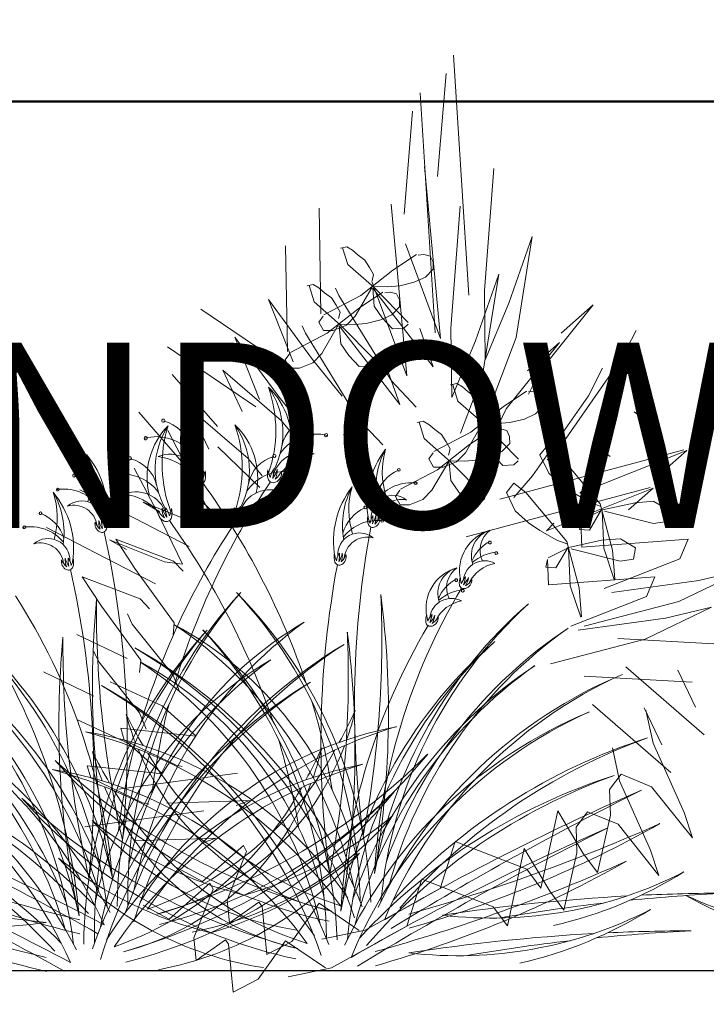
# Model space of a CAD drawing. Units: inches. Extents: x 89 to 490, y -59 to 378.
# Tile 10 of 20: x 352 to 374, y -24 to 7. Entities that reach past the tile are written whole.
import ezdxf

# ---------------------------------------------------------------- set-up
doc = ezdxf.new("R2010")
doc.units = ezdxf.units.IN
doc.header["$MEASUREMENT"] = 0
for name, color, linetype, lineweight in [('A-ANNO-DIMS', 2, 'Continuous', 18), ('L-PLNT', 94, 'Continuous', 18), ('L-PLNT-EDGE', 31, 'Continuous', 25), ('Outer Walls', 12, 'Continuous', 50), ('Windows', 171, 'Continuous', 25)]:
    doc.layers.add(name, color=color, linetype=linetype, lineweight=lineweight)
doc.layers.add('fl', color=73, linetype='Continuous', lineweight=9, true_color=0xa3d166)
doc.styles.get("Standard").update_dxf_attribs({"font": 'arial.ttf'})
doc.dimstyles.get("Standard").update_dxf_attribs({"dimtxt": 6, "dimasz": 4, "dimexe": 3, "dimexo": 3, "dimgap": 0.09, "dimtad": 0, "dimtih": 1, "dimtoh": 1, "dimdec": 1, "dimzin": 0, "dimdsep": 46, "dimlunit": 3, "dimtxsty": 'Standard', "dimcen": 0.09, "dimadec": 0, "dimazin": 0, "dimtfac": 1, "dimtdec": 1, "dimtofl": 0, "dimtmove": 0, "dimatfit": 3, "dimfxl": 1, "dimtolj": 1, "dimtzin": 0, "dimarcsym": 0})

# ---------------------------------------------------------------- blocks, each defined once
blk = doc.blocks.new('Window')
blk.add_lwpolyline([(588.369, 99.053), (588.369, 90.053), (516.369, 90.053), (516.369, 99.053)], close=True)
blk = doc.blocks.new('Plantation')
at = {"layer": 'fl'}
for p, q in [((590.053, 41.103), (590.545, 33.342)), ((589.537, 37.183), (589.811, 40.515)), ((588.969, 39.885), (589.462, 32.124)), ((588.453, 35.965), (588.728, 39.297)), ((589.116, 37.508), (589.628, 31.944)), ((591.356, 37.436), (591.053, 33.489)), ((585.761, 32.741), (585.701, 36.153)), ((588.032, 36.29), (588.545, 30.726)), ((590.272, 36.218), (589.969, 32.271)), ((591.845, 33.078), (592.598, 35.243)), ((592.598, 35.243), (592.077, 31.968)), ((584.677, 31.523), (584.617, 34.935)), ((586.397, 34.862), (586.597, 34.902)), ((586.465, 34.869), (586.629, 34.339)), ((586.597, 34.902), (586.781, 34.796)), ((586.781, 34.796), (586.965, 34.635)), ((589.628, 31.944), (588.494, 35.002)), ((586.965, 34.635), (587.187, 34.475)), ((587.187, 34.475), (587.336, 34.241)), ((588.094, 34.146), (588.854, 34.658)), ((589.094, 34.654), (588.912, 34.633)), ((589.295, 34.603), (589.094, 34.654)), ((589.389, 34.405), (589.295, 34.603)), ((586.629, 34.339), (587.481, 33.591)), ((587.052, 33.333), (588.094, 34.146)), ((587.336, 34.241), (587.468, 34.007)), ((589.143, 33.927), (589.393, 34.186)), ((589.393, 34.186), (589.389, 34.405)), ((588.545, 30.726), (587.411, 33.784)), ((587.468, 34.007), (587.417, 33.806)), ((588.782, 33.757), (589.143, 33.927)), ((590.761, 31.86), (591.514, 34.025)), ((591.514, 34.025), (590.994, 30.75)), ((585.314, 33.644), (585.513, 33.684)), ((585.381, 33.651), (585.545, 33.121)), ((585.513, 33.684), (585.697, 33.578)), ((585.697, 33.578), (585.882, 33.417)), ((586.238, 33.567), (586.343, 33.328)), ((586.872, 32.667), (587.42, 33.605)), ((587.439, 33.569), (589.395, 31.025)), ((587.439, 33.569), (587.485, 32.988)), ((587.474, 33.625), (587.929, 33.614)), ((587.481, 33.591), (588.589, 32.462)), ((587.929, 33.614), (588.311, 33.639)), ((588.311, 33.639), (588.782, 33.757)), ((591.053, 33.489), (591.081, 31.253)), ((584.861, 31.187), (584.063, 33.202)), ((584.063, 33.202), (585.49, 31.257)), ((585.858, 32.709), (587.052, 33.333)), ((585.882, 33.417), (586.103, 33.257)), ((586.103, 33.257), (586.252, 33.023)), ((586.343, 33.328), (588.042, 30.566)), ((587.01, 32.928), (587.77, 33.44)), ((588.01, 33.436), (587.828, 33.415)), ((588.211, 33.385), (588.01, 33.436)), ((588.305, 33.187), (588.211, 33.385)), ((588.309, 32.968), (588.305, 33.187)), ((584.741, 30.944), (581.881, 32.89)), ((585.545, 33.121), (586.397, 32.373)), ((585.968, 32.115), (587.01, 32.928)), ((586.252, 33.023), (586.384, 32.789)), ((587.485, 32.988), (587.747, 32.61)), ((588.059, 32.709), (588.309, 32.968)), ((591.081, 31.253), (591.845, 33.078)), ((594.569, 33.025), (592.844, 30.876)), ((593.531, 32.115), (594.569, 33.025)), ((585.835, 32.667), (585.693, 32.465)), ((586.384, 32.789), (586.333, 32.588)), ((586.587, 32.371), (586.872, 32.667)), ((587.227, 32.421), (587.698, 32.539)), ((587.698, 32.539), (588.059, 32.709)), ((587.747, 32.61), (588.08, 32.251)), ((585.154, 32.349), (585.259, 32.11)), ((585.693, 32.465), (585.844, 32.194)), ((585.789, 31.449), (586.336, 32.387)), ((585.844, 32.194), (586.153, 32.199)), ((586.153, 32.199), (586.587, 32.371)), ((586.355, 32.351), (588.311, 29.807)), ((586.355, 32.351), (586.402, 31.77)), ((586.39, 32.407), (586.845, 32.396)), ((586.397, 32.373), (587.505, 31.244)), ((586.845, 32.396), (587.227, 32.421)), ((588.08, 32.251), (588.444, 32.276)), ((588.444, 32.276), (588.587, 32.406)), ((589.395, 31.025), (588.958, 32.265)), ((589.969, 32.271), (589.997, 30.035)), ((595.959, 32.197), (595.503, 31.307)), ((583.777, 29.969), (582.979, 31.984)), ((582.979, 31.984), (584.406, 30.039)), ((584.774, 31.491), (585.968, 32.115)), ((585.259, 32.11), (586.958, 29.348)), ((592.077, 31.968), (591.363, 30.096)), ((583.658, 29.726), (580.797, 31.672)), ((586.402, 31.77), (586.663, 31.392)), ((589.997, 30.035), (590.761, 31.86)), ((593.485, 31.807), (591.76, 29.658)), ((592.447, 30.897), (593.485, 31.807)), ((584.752, 31.449), (584.61, 31.247)), ((584.61, 31.247), (584.76, 30.976)), ((585.49, 31.257), (586.454, 30.075)), ((585.503, 31.153), (585.789, 31.449)), ((586.663, 31.392), (586.997, 31.033)), ((595.503, 31.307), (593.695, 28.717)), ((583.214, 29.575), (582.585, 30.915)), ((582.585, 30.915), (584.488, 29.278)), ((584.76, 30.976), (585.069, 30.981)), ((585.069, 30.981), (585.503, 31.153)), ((586.997, 31.033), (587.36, 31.058)), ((587.36, 31.058), (587.503, 31.188)), ((588.311, 29.807), (587.874, 31.047)), ((594.875, 30.979), (594.419, 30.089)), ((580.949, 30.771), (582.414, 29.091)), ((590.994, 30.75), (590.28, 28.878)), ((592.844, 30.876), (592.48, 30.134)), ((588.042, 30.566), (588.848, 29.719)), ((589.96, 30.439), (590.159, 30.479)), ((590.027, 30.445), (590.191, 29.916)), ((590.159, 30.479), (590.343, 30.373)), ((590.343, 30.373), (590.528, 30.212)), ((584.406, 30.039), (585.37, 28.857)), ((590.528, 30.212), (590.749, 30.052)), ((590.749, 30.052), (590.898, 29.818)), ((591.656, 29.723), (592.416, 30.235)), ((592.656, 30.231), (592.474, 30.21)), ((594.419, 30.089), (592.611, 27.499)), ((592.857, 30.18), (592.656, 30.231)), ((592.951, 29.982), (592.857, 30.18)), ((592.955, 29.763), (592.951, 29.982)), ((582.13, 28.357), (581.501, 29.697)), ((581.501, 29.697), (583.404, 28.06)), ((590.191, 29.916), (591.043, 29.168)), ((590.614, 28.91), (591.656, 29.723)), ((590.898, 29.818), (591.03, 29.584)), ((591.76, 29.658), (591.396, 28.916)), ((592.705, 29.504), (592.955, 29.763)), ((579.865, 29.553), (581.33, 27.873)), ((586.958, 29.348), (587.765, 28.501)), ((591.03, 29.584), (590.979, 29.383)), ((591.873, 29.216), (592.344, 29.334)), ((592.344, 29.334), (592.705, 29.504)), ((595.902, 29.57), (596.202, 29.338)), ((584.488, 29.278), (584.945, 28.711)), ((588.876, 29.221), (589.075, 29.261)), ((588.943, 29.227), (589.107, 28.698)), ((589.075, 29.261), (589.259, 29.155)), ((589.259, 29.155), (589.444, 28.994)), ((589.444, 28.994), (589.665, 28.834)), ((590.435, 28.244), (590.982, 29.182)), ((590.572, 28.505), (591.332, 29.017)), ((591.001, 29.146), (591.048, 28.564)), ((591.036, 29.202), (591.491, 29.191)), ((591.043, 29.168), (592.151, 28.039)), ((591.572, 29.013), (591.39, 28.992)), ((591.491, 29.191), (591.873, 29.216)), ((591.773, 28.962), (591.572, 29.013)), ((581.532, 27.573), (580.805, 28.958)), ((589.107, 28.698), (589.959, 27.95)), ((589.42, 28.286), (590.614, 28.91)), ((589.665, 28.834), (589.814, 28.6)), ((591.867, 28.764), (591.773, 28.962)), ((591.871, 28.545), (591.867, 28.764)), ((593.695, 28.717), (593.087, 28.016)), ((582.427, 28.43), (583.784, 27.115)), ((589.53, 27.692), (590.572, 28.505)), ((589.814, 28.6), (589.946, 28.366)), ((589.946, 28.366), (589.895, 28.165)), ((591.048, 28.564), (591.309, 28.187)), ((591.621, 28.286), (591.871, 28.545)), ((592.85, 28.177), (593.091, 28.479)), ((593.091, 28.479), (593.481, 28.173)), ((583.404, 28.06), (583.861, 27.493)), ((589.398, 28.244), (589.256, 28.042)), ((589.256, 28.042), (589.406, 27.771)), ((590.149, 27.948), (590.435, 28.244)), ((590.789, 27.998), (591.26, 28.116)), ((591.26, 28.116), (591.621, 28.286)), ((591.309, 28.187), (591.643, 27.828)), ((597.505, 28.338), (591.548, 26.737)), ((593.134, 27.583), (592.85, 28.177)), ((594.798, 26.589), (593.475, 28.174)), ((594.145, 26.934), (597.598, 28.316)), ((594.818, 28.352), (595.118, 28.12)), ((597.598, 28.316), (596.796, 27.608)), ((580.449, 26.355), (579.721, 27.74)), ((589.351, 27.026), (589.898, 27.964)), ((589.406, 27.771), (589.715, 27.776)), ((589.715, 27.776), (590.149, 27.948)), ((589.917, 27.928), (589.964, 27.346)), ((589.953, 27.984), (590.408, 27.973)), ((589.959, 27.95), (591.067, 26.821)), ((590.408, 27.973), (590.789, 27.998)), ((591.643, 27.828), (592.006, 27.853)), ((592.006, 27.853), (592.149, 27.983)), ((582.369, 25.852), (581.532, 27.573)), ((588.336, 27.068), (589.53, 27.692)), ((592.611, 27.499), (592.003, 26.798)), ((593.56, 27.19), (593.134, 27.583)), ((581.343, 27.212), (582.7, 25.897)), ((589.964, 27.346), (590.225, 26.969)), ((596.421, 27.12), (590.464, 25.519)), ((591.766, 26.959), (592.007, 27.261)), ((592.007, 27.261), (592.397, 26.955)), ((593.061, 25.716), (596.514, 27.098)), ((593.934, 26.948), (593.56, 27.19)), ((594.379, 27.185), (594.145, 26.934)), ((596.514, 27.098), (595.712, 26.39)), ((581.495, 25.213), (577.963, 27.037)), ((588.314, 27.026), (588.172, 26.824)), ((588.172, 26.824), (588.322, 26.553)), ((589.065, 26.73), (589.351, 27.026)), ((590.225, 26.969), (590.559, 26.61)), ((590.922, 26.635), (591.065, 26.765)), ((592.05, 26.365), (591.766, 26.959)), ((593.714, 25.371), (592.391, 26.956)), ((594.479, 26.634), (593.934, 26.948)), ((580.554, 26.325), (580.008, 26.646)), ((580.008, 26.646), (581.783, 25.929)), ((588.322, 26.553), (588.631, 26.558)), ((588.631, 26.558), (589.065, 26.73)), ((590.559, 26.61), (590.922, 26.635)), ((594.803, 26.513), (594.479, 26.634)), ((595.202, 25.087), (594.798, 26.589)), ((595.927, 26.626), (594.873, 26.397)), ((596.534, 26.679), (595.927, 26.626)), ((596.536, 26.669), (597.02, 26.38)), ((581.285, 24.634), (580.449, 26.355)), ((592.476, 25.972), (592.05, 26.365)), ((594.873, 26.397), (594.195, 26.057)), ((594.451, 25.739), (594.846, 26.409)), ((594.913, 25.157), (594.86, 26.374)), ((596.526, 25.953), (594.938, 26.356)), ((597.02, 26.38), (596.956, 26.019)), ((580.411, 23.995), (576.879, 25.819)), ((581.783, 25.929), (582.369, 25.852)), ((592.85, 25.73), (592.476, 25.972)), ((593.296, 25.967), (593.061, 25.716)), ((594.176, 26.011), (594.128, 25.758)), ((594.176, 26.011), (594.205, 25.186)), ((596.956, 26.019), (596.526, 25.953)), ((593.395, 25.416), (592.85, 25.73)), ((594.128, 25.758), (594.451, 25.739)), ((579.47, 25.107), (578.925, 25.428)), ((578.925, 25.428), (580.699, 24.711)), ((579.741, 24.498), (579.126, 25.45)), ((579.126, 25.45), (580.997, 24.736)), ((593.789, 25.179), (593.111, 24.839)), ((593.367, 24.521), (593.762, 25.191)), ((593.719, 25.295), (593.395, 25.416)), ((594.119, 23.869), (593.714, 25.371)), ((594.844, 25.408), (593.789, 25.179)), ((594.205, 25.186), (597.647, 25.449)), ((595.45, 25.461), (594.844, 25.408)), ((595.452, 25.451), (595.936, 25.162)), ((597.647, 25.449), (597.377, 24.808)), ((593.83, 23.939), (593.776, 25.156)), ((595.442, 24.735), (593.855, 25.138)), ((595.251, 24.138), (594.913, 25.157)), ((595.273, 24.155), (595.202, 25.087)), ((595.936, 25.162), (595.872, 24.801)), ((580.699, 24.711), (581.285, 24.634)), ((580.997, 24.736), (581.3, 24.406)), ((593.093, 24.793), (593.044, 24.54)), ((593.044, 24.54), (593.367, 24.521)), ((593.093, 24.793), (593.121, 23.968)), ((597.377, 24.808), (594.931, 23.85)), ((595.872, 24.801), (595.442, 24.735)), ((578.658, 23.28), (578.042, 24.232)), ((578.042, 24.232), (579.913, 23.518)), ((581.017, 22.743), (579.741, 24.498)), ((593.121, 23.968), (596.563, 24.231)), ((596.563, 24.231), (596.293, 23.59)), ((599.485, 24.463), (597.342, 23.428)), ((597.995, 24.105), (599.485, 24.463)), ((594.167, 22.92), (593.83, 23.939)), ((595.175, 23.723), (597.995, 24.105)), ((596.293, 23.59), (593.847, 22.632)), ((594.189, 22.937), (594.119, 23.869)), ((579.933, 21.525), (578.658, 23.28)), ((579.913, 23.518), (580.216, 23.188)), ((597.342, 23.428), (594.28, 22.626)), ((579.657, 22.697), (579.5, 23.032)), ((598.401, 23.245), (596.258, 22.21)), ((596.911, 22.887), (598.401, 23.245)), ((580.977, 21.04), (579.657, 22.697)), ((580.981, 22.353), (581.017, 22.743)), ((594.091, 22.505), (596.911, 22.887)), ((577.865, 22.366), (579.494, 21.586)), ((596.258, 22.21), (593.196, 21.408)), ((595.368, 22.229), (598.862, 22.04)), ((578.573, 21.479), (578.416, 21.814)), ((579.894, 19.822), (578.573, 21.479)), ((579.897, 21.135), (579.933, 21.525)), ((576.781, 21.148), (578.41, 20.368)), ((581.19, 20.513), (580.977, 21.04)), ((595.633, 21.318), (598.165, 19.117)), ((597.306, 21.208), (597.881, 20.013)), ((580.622, 20.056), (578.943, 20.825)), ((594.284, 21.011), (597.778, 20.822)), ((594.549, 20.1), (597.081, 17.899)), ((580.106, 19.295), (579.894, 19.822)), ((581.725, 19.073), (580.622, 20.056)), ((596.222, 19.99), (596.797, 18.795)), ((596.28, 19.909), (596.511, 18.848)), ((579.538, 18.838), (577.859, 19.607)), ((579.396, 18.945), (579.286, 19.33)), ((579.286, 19.33), (580.993, 19.145)), ((580.993, 19.145), (581.725, 19.073)), ((581.077, 18.127), (579.396, 18.945)), ((580.641, 17.855), (579.538, 18.838)), ((596.511, 18.848), (597.511, 16.597)), ((595.196, 18.691), (595.427, 17.63)), ((578.312, 17.727), (578.202, 18.112)), ((578.202, 18.112), (579.91, 17.927)), ((579.208, 17.36), (583.059, 17.877)), ((579.91, 17.927), (580.641, 17.855)), ((581.273, 18.085), (581.077, 18.127)), ((579.993, 16.909), (578.312, 17.727)), ((595.476, 17.84), (595.104, 17.341)), ((595.427, 17.63), (596.428, 15.379)), ((596.462, 17.436), (595.476, 17.84)), ((595.104, 17.341), (595.132, 16.516)), ((597.782, 15.78), (596.462, 17.436)), ((580.189, 16.867), (579.993, 16.909)), ((582.478, 16.96), (580.778, 16.902)), ((583.449, 16.993), (582.478, 16.96)), ((583.017, 16.832), (583.449, 16.993)), ((578.125, 16.142), (581.975, 16.659)), ((593.426, 16.652), (592.879, 14.154)), ((594.251, 15.271), (593.426, 16.652)), ((594.392, 16.622), (594.02, 16.123)), ((595.378, 16.218), (594.392, 16.622)), ((597.511, 16.597), (597.782, 15.78)), ((595.132, 16.516), (594.709, 14.654)), ((594.02, 16.123), (594.048, 15.298)), ((596.698, 14.562), (595.378, 16.218)), ((581.394, 15.741), (579.694, 15.684)), ((582.365, 15.775), (581.394, 15.741)), ((581.933, 15.614), (582.365, 15.775)), ((590.105, 15.664), (589.623, 14.141)), ((592.421, 14.771), (590.105, 15.664)), ((583.256, 15.528), (581.934, 14.365)), ((582.733, 13.76), (583.359, 15.337)), ((583.359, 15.337), (583.256, 15.528)), ((592.342, 15.434), (591.795, 12.936)), ((593.167, 14.053), (592.342, 15.434)), ((594.048, 15.298), (593.626, 13.436)), ((596.428, 15.379), (596.698, 14.562)), ((594.709, 14.654), (594.251, 15.271)), ((581.934, 14.365), (581.092, 14.822)), ((592.879, 14.154), (592.421, 14.771)), ((589.022, 14.446), (588.539, 12.923)), ((591.337, 13.553), (589.022, 14.446)), ((582.172, 14.31), (580.85, 13.146)), ((581.649, 12.542), (582.276, 14.119)), ((582.276, 14.119), (582.172, 14.31)), ((589.623, 14.141), (587.189, 12.794)), ((593.626, 13.436), (593.167, 14.053)), ((582.806, 13.033), (582.733, 13.76)), ((580.85, 13.146), (580.008, 13.604)), ((583.756, 13.697), (582.806, 13.033)), ((583.858, 13.555), (583.756, 13.697)), ((584.008, 12.005), (583.858, 13.555)), ((585.701, 13.667), (584.82, 12.421)), ((586.995, 12.787), (585.701, 13.667)), ((591.795, 12.936), (591.337, 13.553)), ((587.189, 12.794), (585.79, 12.503)), ((588.539, 12.923), (586.106, 11.576)), ((581.722, 11.815), (581.649, 12.542)), ((582.672, 12.479), (581.722, 11.815)), ((582.774, 12.337), (582.672, 12.479)), ((584.617, 12.449), (583.736, 11.203)), ((585.911, 11.569), (584.617, 12.449)), ((582.924, 10.787), (582.774, 12.337)), ((584.82, 12.421), (584.008, 12.005)), ((586.106, 11.576), (584.706, 11.285)), ((583.736, 11.203), (582.924, 10.787))]:
    blk.add_line(p, q, dxfattribs=at)
for centre, radius, start, end in [((583.596, 28.668), 2.375, 135.5632, 193.7293), ((584.084, 28.918), 2.601, 147.096, 209.2874), ((585.935, 29.073), 4.227, 162.6858, 201.1197), ((581.93, 28.875), 2.601, 332.7126, 34.904), ((582.427, 28.642), 2.375, 348.2707, 46.4368), ((580.075, 28.965), 4.227, 340.8803, 19.3142), ((580.662, 29.279), 0.053, 11.802, 191.802), ((585.639, 28.222), 1.163, 105.8563, 168.2872), ((585.338, 29.356), 0.053, 350.198, 170.198), ((585.338, 29.356), 0.053, 170.198, 350.198), ((582.512, 27.45), 2.375, 135.5632, 193.7293), ((583, 27.7), 2.601, 147.096, 209.2874), ((580.662, 29.279), 0.053, 191.802, 11.802), ((584.851, 27.855), 4.227, 162.6858, 201.1197), ((580.4, 28.136), 1.163, 13.7128, 76.1437), ((580.847, 27.657), 2.601, 332.7126, 34.904), ((581.343, 27.424), 2.375, 348.2707, 46.4368), ((578.991, 27.747), 4.227, 340.8803, 19.3142), ((580.093, 28.713), 0.053, 11.802, 191.802), ((580.441, 27.347), 1.416, 35.6636, 106.404), ((580.093, 28.713), 0.053, 191.802, 11.802), ((585.626, 27.432), 1.416, 75.596, 146.3364), ((585.925, 28.809), 0.053, 170.198, 350.198), ((585.925, 28.809), 0.053, 350.198, 170.198), ((575.991, 26.352), 2.854, 351.4134, 39.8275), ((575.706, 27.362), 2.608, 344.3064, 18.279), ((575.935, 26.873), 2.6, 351.5096, 30.1949), ((579.578, 28.061), 0.053, 11.802, 191.802), ((579.578, 28.061), 0.053, 191.802, 11.802), ((579.316, 26.918), 1.163, 13.7128, 76.1437), ((580.873, 27.183), 1.01, 11.1862, 111.7493), ((580.216, 26.257), 1.886, 44.0209, 81.3627), ((584.555, 27.004), 1.163, 105.8563, 168.2872), ((584.254, 28.138), 0.053, 350.198, 170.198), ((584.254, 28.138), 0.053, 170.198, 350.198), ((585.199, 27.253), 1.01, 70.2507, 170.8138), ((585.889, 26.351), 1.886, 100.6373, 137.9791), ((590.108, 26.604), 2.854, 142.1725, 190.5866), ((590.145, 27.126), 2.6, 151.8051, 190.4904), ((590.357, 27.623), 2.608, 163.721, 197.6936), ((588.284, 27.691), 0.0459, 354.4108, 174.4108), ((577.775, 27.502), 0.0459, 7.5892, 187.5892), ((577.775, 27.502), 0.0459, 187.5892, 7.5892), ((577.34, 26.331), 1.243, 16.8512, 68.8014), ((579.009, 27.495), 0.053, 11.802, 191.802), ((579.357, 26.129), 1.416, 35.6636, 106.404), ((579.009, 27.495), 0.053, 191.802, 11.802), ((581.906, 27.557), 0.334, 172.3781, 246.6066), ((582.195, 27.901), 0.689, 205.7422, 233.1344), ((582.36, 27.654), 0.654, 178.723, 207.7572), ((582.516, 27.921), 0.848, 197.3111, 219.7508), ((581.179, 27.188), 0.803, 16.3461, 37.9549), ((583.321, 27.787), 1.513, 184.0141, 195.6693), ((580.816, 27.847), 1.213, 339.0728, 350.8866), ((581.342, 27.507), 0.688, 348.1534, 12.4334), ((584.542, 26.214), 1.416, 75.596, 146.3364), ((584.72, 27.56), 0.688, 169.5666, 193.8466), ((585.233, 27.919), 1.213, 191.1134, 202.9272), ((584.894, 27.247), 0.803, 144.0451, 165.6539), ((582.732, 27.772), 1.513, 346.3307, 357.9859), ((583.531, 27.933), 0.848, 322.2492, 344.6889), ((583.697, 27.672), 0.654, 334.2428, 3.277), ((583.853, 27.925), 0.689, 308.8656, 336.2578), ((584.154, 27.591), 0.334, 295.3934, 9.6219), ((584.841, 27.591), 0.053, 170.198, 350.198), ((584.841, 27.591), 0.053, 350.198, 170.198), ((588.76, 26.535), 1.243, 113.1986, 165.1488), ((588.284, 27.691), 0.0459, 174.4108, 354.4108), ((577.249, 27.05), 0.0459, 7.5892, 187.5892), ((604.656, 13.567), 24.696, 146.2244, 163.2125), ((581.846, 27.41), 0.175, 245.3588, 345.3239), ((561.906, 12.826), 24.696, 18.7875, 35.7756), ((584.219, 27.446), 0.175, 196.6761, 296.6412), ((589.024, 25.386), 2.854, 142.1725, 190.5866), ((589.061, 25.908), 2.6, 151.8051, 190.4904), ((589.273, 26.405), 2.608, 163.721, 197.6936), ((588.675, 25.883), 1.386, 81.8677, 142.4931), ((588.826, 27.257), 0.0459, 354.4108, 174.4108), ((588.826, 27.257), 0.0459, 174.4108, 354.4108), ((574.907, 25.134), 2.854, 351.4134, 39.8275), ((574.622, 26.144), 2.608, 344.3064, 18.279), ((574.851, 25.654), 2.6, 351.5096, 30.1949), ((577.447, 25.682), 1.386, 39.5069, 100.1323), ((577.249, 27.05), 0.0459, 187.5892, 7.5892), ((579.789, 25.965), 1.01, 11.1862, 111.7493), ((579.132, 25.039), 1.886, 44.0209, 81.3627), ((584.115, 26.035), 1.01, 70.2507, 170.8138), ((584.805, 25.132), 1.886, 100.6373, 137.9791), ((588.092, 26.164), 0.701, 51.1297, 184.5825), ((578.02, 25.984), 0.701, 357.4175, 130.8703), ((577.77, 25.789), 0.754, 6.9832, 106.1055), ((581.276, 26.436), 0.654, 178.723, 207.7572), ((581.432, 26.703), 0.848, 197.3111, 219.7508), ((580.095, 25.97), 0.803, 16.3461, 37.9549), ((582.237, 26.569), 1.513, 184.0141, 195.6693), ((583.636, 26.342), 0.688, 169.5666, 193.8466), ((584.149, 26.701), 1.213, 191.1134, 202.9272), ((583.81, 26.029), 0.803, 144.0451, 165.6539), ((581.648, 26.554), 1.513, 346.3307, 357.9859), ((582.448, 26.715), 0.848, 322.2492, 344.6889), ((582.613, 26.454), 0.654, 334.2428, 3.277), ((587.676, 25.317), 1.243, 113.1986, 165.1488), ((587.2, 26.473), 0.0459, 174.4108, 354.4108), ((587.2, 26.473), 0.0459, 354.4108, 174.4108), ((588.349, 25.979), 0.754, 75.8945, 175.0168), ((576.691, 26.284), 0.0459, 7.5892, 187.5892), ((576.691, 26.284), 0.0459, 187.5892, 7.5892), ((576.256, 25.113), 1.243, 16.8512, 68.8014), ((580.822, 26.339), 0.334, 172.3781, 246.6066), ((581.112, 26.683), 0.689, 205.7422, 233.1344), ((580.762, 26.192), 0.175, 245.3588, 345.3239), ((579.732, 26.629), 1.213, 339.0728, 350.8866), ((580.258, 26.289), 0.688, 348.1534, 12.4334), ((583.135, 26.228), 0.175, 196.6761, 296.6412), ((582.769, 26.707), 0.689, 308.8656, 336.2578), ((583.07, 26.373), 0.334, 295.3934, 9.6219), ((587.865, 26.103), 0.595, 173.7794, 198.0594), ((588.285, 26.445), 1.049, 195.3262, 207.14), ((588.035, 25.844), 0.694, 148.2579, 169.8667), ((586.138, 26.159), 1.308, 350.5435, 2.1987), ((586.817, 26.35), 0.733, 326.462, 348.9017), ((586.976, 26.135), 0.565, 338.4556, 7.4897), ((587.095, 26.363), 0.596, 313.0784, 340.4706), ((587.376, 26.094), 0.289, 299.6062, 13.8346), ((576.165, 25.832), 0.0459, 7.5892, 187.5892), ((576.363, 24.464), 1.386, 39.5069, 100.1323), ((576.165, 25.832), 0.0459, 187.5892, 7.5892), ((578.739, 25.938), 0.289, 168.1654, 242.3938), ((579.01, 26.216), 0.596, 201.5294, 228.9216), ((579.137, 25.993), 0.565, 174.5103, 203.5444), ((579.288, 26.213), 0.733, 193.0983, 215.538), ((579.974, 26.047), 1.308, 179.8013, 191.4565), ((578.088, 25.666), 0.694, 12.1333, 33.7421), ((577.817, 26.257), 1.049, 334.86, 346.6738), ((578.249, 25.93), 0.595, 343.9406, 8.2206), ((603.572, 12.349), 24.696, 146.2244, 163.2125), ((560.822, 11.608), 24.696, 18.7875, 35.7756), ((587.591, 24.665), 1.386, 81.8677, 142.4931), ((618.338, 20.073), 31.492, 169.4573, 187.7209), ((587.441, 25.973), 0.151, 200.8889, 300.854), ((587.742, 26.039), 0.0459, 354.4108, 174.4108), ((587.742, 26.039), 0.0459, 174.4108, 354.4108), ((578.678, 25.815), 0.151, 241.146, 341.1111), ((548.006, 18.841), 31.492, 354.2791, 12.5427), ((587.008, 24.946), 0.701, 51.1297, 184.5825), ((587.265, 24.761), 0.754, 75.8945, 175.0168), ((591.615, 24.421), 1.368, 105.8634, 192.367), ((591.493, 24.911), 0.863, 106.9799, 199.184), ((591.704, 25.093), 0.793, 125.7722, 206.2024), ((576.936, 24.766), 0.701, 357.4175, 130.8703), ((576.687, 24.571), 0.754, 6.9832, 106.1055), ((591.8, 24.269), 1.243, 116.6992, 157.9158), ((591.227, 25.335), 0.0459, 162.351, 342.351), ((591.227, 25.335), 0.0459, 342.351, 162.351), ((586.781, 24.885), 0.595, 173.7794, 198.0594), ((587.202, 25.227), 1.049, 195.3262, 207.14), ((586.951, 24.626), 0.694, 148.2579, 169.8667), ((585.054, 24.941), 1.308, 350.5435, 2.1987), ((585.733, 25.132), 0.733, 326.462, 348.9017), ((585.892, 24.917), 0.565, 338.4556, 7.4897), ((586.011, 25.145), 0.596, 313.0784, 340.4706), ((586.292, 24.876), 0.289, 299.6062, 13.8346), ((591.58, 23.649), 1.386, 94.6451, 131.584), ((591.438, 24.996), 0.0459, 162.351, 342.351), ((591.438, 24.996), 0.0459, 342.351, 162.351), ((577.655, 24.72), 0.289, 168.1654, 242.3938), ((577.927, 24.998), 0.596, 201.5294, 228.9216), ((578.053, 24.775), 0.565, 174.5103, 203.5444), ((578.204, 24.995), 0.733, 193.0983, 215.538), ((577.594, 24.597), 0.151, 241.146, 341.1111), ((578.89, 24.829), 1.308, 179.8013, 191.4565), ((577.005, 24.448), 0.694, 12.1333, 33.7421), ((576.734, 25.039), 1.049, 334.86, 346.6738), ((577.165, 24.712), 0.595, 343.9406, 8.2206), ((617.254, 18.855), 31.492, 169.4573, 187.7209), ((586.357, 24.755), 0.151, 200.8889, 300.854), ((591.064, 24.05), 0.696, 61.775, 172.7958), ((591.598, 23.527), 1.154, 100.1929, 154.0707), ((546.922, 17.622), 31.492, 354.2791, 12.5427), ((590.531, 23.203), 1.368, 105.8634, 192.367), ((590.409, 23.693), 0.863, 106.9799, 199.184), ((590.621, 23.875), 0.793, 125.7722, 206.2024), ((590.834, 24.033), 0.595, 161.7196, 185.9995), ((591.316, 24.28), 1.049, 183.2663, 195.0802), ((590.946, 23.745), 0.694, 136.198, 157.8068), ((589.157, 24.449), 1.308, 338.4836, 350.1389), ((590.716, 23.051), 1.243, 116.6992, 157.9158), ((590.143, 24.117), 0.0459, 162.351, 342.351), ((590.143, 24.117), 0.0459, 342.351, 162.351), ((590.392, 23.994), 0.151, 188.8291, 288.7942), ((589.86, 24.493), 0.733, 314.4022, 336.8418), ((590.354, 24.127), 0.289, 287.5463, 1.7748), ((589.971, 24.25), 0.565, 326.3958, 355.4299), ((590.135, 24.448), 0.596, 301.0185, 328.4108), ((558.885, 12.66), 20.216, 5.151, 32.7872), ((594.374, 13.451), 15.201, 137.4916, 179.6099), ((594.436, 13.941), 14.921, 139.0392, 181.297), ((572.107, 13.556), 14.921, 0.703, 42.9608), ((572.186, 13.068), 15.201, 2.3901, 44.5084), ((553.743, 22.201), 33.989, 349.2183, 2.4529), ((607.681, 13.517), 20.216, 149.2128, 176.849), ((558.054, 19.814), 29.894, 350.0105, 7.3826), ((590.497, 22.431), 1.386, 94.6451, 131.584), ((590.354, 23.777), 0.0459, 162.351, 342.351), ((590.354, 23.777), 0.0459, 342.351, 162.351), ((608.262, 20.685), 29.894, 174.6174, 191.9895), ((612.487, 23.221), 33.989, 179.5471, 192.7817), ((602.446, 11.881), 15.201, 130.9977, 169.5878), ((602.563, 12.361), 14.921, 132.5453, 174.8032), ((589.981, 22.832), 0.696, 61.775, 172.7958), ((590.514, 22.309), 1.154, 100.1929, 154.0707), ((564.04, 11.683), 14.921, 7.1968, 49.4547), ((564.174, 11.208), 15.201, 12.4122, 51.0023), ((589.75, 22.815), 0.595, 161.7196, 185.9995), ((590.233, 23.062), 1.049, 183.2663, 195.0802), ((589.862, 22.527), 0.694, 136.198, 157.8068), ((588.073, 23.231), 1.308, 338.4836, 350.1389), ((588.777, 23.275), 0.733, 314.4022, 336.8418), ((588.887, 23.032), 0.565, 326.3958, 355.4299), ((591.294, 12.388), 12.017, 120.3536, 167.8423), ((593.323, 11.517), 13.856, 125.7805, 169.1581), ((573.304, 11.172), 13.856, 12.8419, 56.2195), ((575.301, 12.114), 12.017, 14.1577, 61.6464), ((606.597, 12.299), 20.216, 149.2128, 176.849), ((589.308, 22.776), 0.151, 188.8291, 288.7942), ((589.27, 22.909), 0.289, 287.5463, 1.7748), ((589.051, 23.23), 0.596, 301.0185, 328.4108), ((557.801, 11.442), 20.216, 5.151, 32.7872), ((593.29, 12.232), 15.201, 137.4916, 179.6099), ((593.352, 12.723), 14.921, 139.0392, 181.297), ((571.023, 12.338), 14.921, 0.703, 42.9608), ((571.102, 11.85), 15.201, 2.3901, 44.5084), ((552.659, 20.983), 33.989, 349.2183, 2.4529), ((556.97, 18.596), 29.894, 350.0105, 7.3826), ((602.203, 9.926), 15.201, 123.7186, 160.4349), ((602.38, 10.388), 14.921, 125.2661, 165.1679), ((564.292, 9.718), 14.921, 16.8321, 56.7339), ((564.484, 9.263), 15.201, 21.5651, 58.2814), ((607.178, 19.467), 29.894, 174.6174, 191.9895), ((611.403, 22.003), 33.989, 179.5471, 192.7817), ((595.117, 7.795), 16.642, 121.1471, 160.292), ((595.251, 8.353), 16.239, 122.567, 163.1344), ((601.362, 10.663), 15.201, 130.9977, 169.5878), ((601.479, 11.143), 14.921, 132.5453, 174.8032), ((562.957, 10.465), 14.921, 7.1968, 49.4547), ((563.09, 9.99), 15.201, 12.4122, 51.0023), ((571.64, 7.391), 16.642, 21.708, 60.8529), ((571.487, 7.943), 16.239, 18.8656, 59.433), ((590.21, 11.17), 12.017, 120.3536, 167.8423), ((592.239, 10.299), 13.856, 125.7805, 169.1581), ((572.22, 9.954), 13.856, 12.8419, 56.2195), ((574.217, 10.896), 12.017, 14.1577, 61.6464), ((601.12, 8.708), 15.201, 123.7186, 160.4349), ((601.296, 9.17), 14.921, 125.2661, 165.1679), ((601.359, 7.034), 15.201, 112.5744, 154.7193), ((601.621, 7.453), 14.921, 114.122, 157.6363), ((563.208, 8.5), 14.921, 16.8321, 56.7339), ((563.401, 8.045), 15.201, 21.5651, 58.2814), ((594.034, 6.577), 16.642, 121.1471, 160.292), ((594.167, 7.135), 16.239, 122.567, 163.1344), ((565.43, 6.402), 15.201, 27.2807, 69.4256), ((565.153, 6.811), 14.921, 24.3637, 67.878), ((570.556, 6.173), 16.642, 21.708, 60.8529), ((570.404, 6.725), 16.239, 18.8656, 59.433), ((602.195, 14.513), 22.067, 165.3183, 172.932), ((564.333, 13.858), 22.067, 9.068, 16.6817), ((588.037, 22.079), 8.88, 194.9574, 201.3849), ((591.138, 25.442), 12.977, 205.8333, 210.9541), ((575.002, 25.155), 12.977, 331.0459, 336.1667), ((600.275, 5.816), 15.201, 112.5744, 154.7193), ((578.218, 21.902), 8.88, 340.6151, 347.0426), ((600.537, 6.235), 14.921, 114.122, 157.6363), ((564.346, 5.184), 15.201, 27.2807, 69.4256), ((564.069, 5.593), 14.921, 24.3637, 67.878), ((576.177, 6.722), 12.64, 34.1912, 81.04), ((574.36, 4.785), 14.911, 36.1662, 75.2917), ((590.606, 6.968), 12.64, 100.96, 147.8088), ((592.49, 5.097), 14.911, 106.7083, 145.8338), ((601.111, 13.295), 22.067, 165.3183, 172.932), ((563.249, 12.64), 22.067, 9.068, 16.6817), ((602.197, 0.739), 19.194, 107.7857, 137.2506), ((602.811, 0.997), 19.147, 109.7712, 139.1936), ((564.812, 0.081), 19.194, 44.7494, 74.2143), ((564.189, 0.318), 19.147, 42.8064, 72.2288), ((586.953, 20.861), 8.88, 194.9574, 201.3849), ((590.054, 24.224), 12.977, 205.8333, 210.9541), ((588.037, 22.079), 8.88, 202.7107, 257.3947), ((576.513, 23.895), 11.042, 289.2472, 331.4766), ((589.672, 24.13), 11.042, 210.5234, 252.7528), ((578.218, 21.902), 8.88, 284.6053, 339.2893), ((574.743, 32.962), 20.466, 286.2137, 315.0057), ((576.569, 28.812), 16.324, 284.0723, 320.7861), ((573.918, 23.937), 12.977, 331.0459, 336.1667), ((577.134, 20.684), 8.88, 340.6151, 347.0426), ((591.124, 33.253), 20.466, 226.9943, 255.7863), ((589.444, 29.042), 16.324, 221.2139, 257.9277), ((575.094, 5.504), 12.64, 34.1912, 81.04), ((573.276, 3.567), 14.911, 36.1662, 75.2917), ((589.523, 5.75), 12.64, 100.96, 147.8088), ((591.406, 3.879), 14.911, 106.7083, 145.8338), ((577.134, 20.684), 8.88, 284.6053, 339.2893), ((601.113, -0.479), 19.194, 107.7857, 137.2506), ((601.727, -0.221), 19.147, 109.7712, 139.1936), ((563.728, -1.137), 19.194, 44.7494, 74.2143), ((563.105, -0.9), 19.147, 42.8064, 72.2288), ((586.953, 20.861), 8.88, 202.7107, 257.3947), ((575.429, 22.677), 11.042, 289.2472, 331.4766), ((588.588, 22.912), 11.042, 210.5234, 252.7528), ((573.659, 31.744), 20.466, 286.2137, 315.0057), ((575.485, 27.594), 16.324, 284.0723, 320.7861), ((629.196, -58.6), 82.807, 113.53444, 119.97645), ((644.056, -79.126), 107.696, 116.42332, 121.34648), ((590.04, 32.035), 20.466, 226.9943, 255.7863), ((588.361, 27.824), 16.324, 221.2139, 257.9277), ((525.765, -81.196), 107.696, 60.65352, 65.57668), ((539.899, -60.164), 82.807, 62.02355, 68.46556), ((586.476, 26.666), 13.137, 231.8384, 256.0141), ((586.706, 23.991), 11.325, 222.5197, 261.2503), ((579.482, 23.859), 11.325, 280.7497, 319.4803), ((579.618, 26.541), 13.137, 285.9859, 310.1616), ((628.113, -59.818), 82.807, 113.53444, 119.97645), ((642.972, -80.344), 107.696, 116.42332, 121.34648), ((572.899, 69.711), 58.541, 285.56, 294.0219), ((578.638, 48.251), 36.77, 285.7446, 299.4741), ((524.681, -82.414), 107.696, 60.65352, 65.57668), ((538.815, -61.382), 82.807, 62.02355, 68.46556), ((586.697, 48.387), 36.77, 242.5259, 256.2554), ((591.684, 70.033), 58.541, 247.9781, 256.44), ((585.392, 25.448), 13.137, 231.8384, 256.0141), ((585.622, 22.773), 11.325, 222.5197, 261.2503), ((578.398, 22.641), 11.325, 280.7497, 319.4803), ((578.534, 25.323), 13.137, 285.9859, 310.1616), ((571.815, 68.493), 58.541, 285.56, 294.0219), ((577.555, 47.033), 36.77, 285.7446, 299.4741), ((591.286, 26.887), 13.704, 263.3334, 297.0085), ((590.133, 26.627), 14.044, 282.9751, 301.6856), ((585.614, 47.169), 36.77, 242.5259, 256.2554), ((590.6, 68.815), 58.541, 247.9781, 256.44), ((574.803, 26.594), 13.704, 244.9915, 278.6666), ((598.969, -46.365), 60.356, 93.13909, 98.84209), ((601.803, -46.334), 60.398, 92.82762, 95.73925), ((598.969, -46.365), 60.356, 90.13814, 92.7056), ((604.53, 26.12), 14.044, 240.3144, 259.0249), ((603.368, 26.339), 13.704, 244.9915, 278.6666), ((569.681, -46.882), 60.356, 83.15791, 88.86091), ((590.203, 25.669), 13.704, 263.3334, 297.0085), ((601.803, -46.334), 60.398, 96.55624, 99.79042), ((589.049, 25.409), 14.044, 282.9751, 301.6856), ((600.719, -47.552), 60.398, 92.82762, 95.73925), ((597.885, -47.583), 60.356, 90.13814, 92.7056), ((597.885, -47.583), 60.356, 93.13909, 98.84209), ((600.719, -47.552), 60.398, 96.55624, 99.79042)]:
    blk.add_arc(centre, radius, start, end, dxfattribs=at)
blk = doc.blocks.new('*D36')
at = {"layer": 'A-ANNO-DIMS', "color": 0, "lineweight": -2, "transparency": 16777216}
for p, q in [((327.654, 1.741), (327.654, -9.059)), ((399.654, 1.741), (399.654, -9.059)), ((331.654, -6.059), (339.621, -6.059)), ((395.654, -6.059), (387.687, -6.059))]:
    blk.add_line(p, q, dxfattribs=at)
at = {"layer": 'A-ANNO-DIMS', "color": 0, "transparency": 16777216}
for points in [[(331.654, -5.392), (331.654, -6.725), (327.654, -6.059)], [(395.654, -5.392), (395.654, -6.725), (399.654, -6.059)]]:
    blk.add_solid(points, dxfattribs=at)
at = {"layer": 'Defpoints', "color": 0, "transparency": 16777216}
for p in [(327.654, 4.741), (399.654, 4.741), (399.654, -6.059)]:
    blk.add_point(p, dxfattribs=at)
at = {"layer": 'A-ANNO-DIMS', "color": 0, "transparency": 16777216, "insert": (363.654, -6.059), "char_height": 6, "attachment_point": 5}
blk.add_mtext('\\A1;WINDOW 72', dxfattribs=at)
blk = doc.blocks.new('*D48')
at = {"layer": 'A-ANNO-DIMS', "color": 0, "lineweight": -2, "transparency": 16777216}
for p, q in [((127.441, 10.741), (127.441, -49.809)), ((459.441, -29.659), (459.441, -49.809)), ((131.441, -46.809), (286.756, -46.809)), ((455.441, -46.809), (300.127, -46.809))]:
    blk.add_line(p, q, dxfattribs=at)
at = {"layer": 'A-ANNO-DIMS', "color": 0, "transparency": 16777216}
for points in [[(131.441, -46.143), (131.441, -47.476), (127.441, -46.809)], [(455.441, -46.143), (455.441, -47.476), (459.441, -46.809)]]:
    blk.add_solid(points, dxfattribs=at)
at = {"layer": 'Defpoints', "color": 0, "transparency": 16777216}
for p in [(127.441, 13.741), (459.441, -26.659), (459.441, -46.809)]:
    blk.add_point(p, dxfattribs=at)
at = {"layer": 'A-ANNO-DIMS', "color": 0, "transparency": 16777216, "insert": (293.441, -46.809), "char_height": 6, "attachment_point": 5}
blk.add_mtext('\\A1;332', dxfattribs=at)

msp = doc.modelspace()

# ---------------------------------------------------------------- linework, layer by layer
at = {"layer": 'L-PLNT-EDGE'}
msp.add_line((459.4414, -23.3886), (265.4414, -23.3886), dxfattribs=at)
at = {"layer": 'Outer Walls'}
msp.add_lwpolyline([(214.6478, 67.7413), (265.4414, 67.7413), (265.4414, 4.7413), (459.4414, 4.7413), (459.4414, 353.7413), (127.4414, 353.7413), (127.4414, 13.7413)], dxfattribs=at)

# ---------------------------------------------------------------- block references
at = {"layer": 'L-PLNT'}
msp.add_blockref('Plantation', (-223.8856, -34.8668), dxfattribs=at)
at = {"layer": 'Windows'}
msp.add_blockref('Window', (-188.7147, -85.3119), dxfattribs=at)

# ---------------------------------------------------------------- dimensions: what is measured, and where the dimension line sits
at = {"layer": 'A-ANNO-DIMS'}
dim = msp.add_linear_dim(base=(459.4414, -46.8094), p1=(127.4414, 13.7413), p2=(459.4414, -26.6594), dimstyle='Standard', override={"dimdec": 0, "dimlfac": 1, "dimrnd": 0, "dimzin": 0, "dimdsep": 46, "dimlunit": 2}, dxfattribs=at)
dim.commit()
dim.dimension.update_dxf_attribs({"geometry": '*D48', "text_midpoint": (293.4414, -46.8094)})
dim = msp.add_linear_dim(base=(399.6539, -6.0587), p1=(327.6539, 4.7413), p2=(399.6539, 4.7413), text='WINDOW <>', dimstyle='Standard', override={"dimdec": 0, "dimlfac": 1, "dimrnd": 0, "dimzin": 0, "dimdsep": 46, "dimlunit": 2}, dxfattribs=at)
dim.commit()
dim.dimension.update_dxf_attribs({"geometry": '*D36', "text_midpoint": (363.6539, -6.0587)})

doc.saveas('drawing.dxf')
